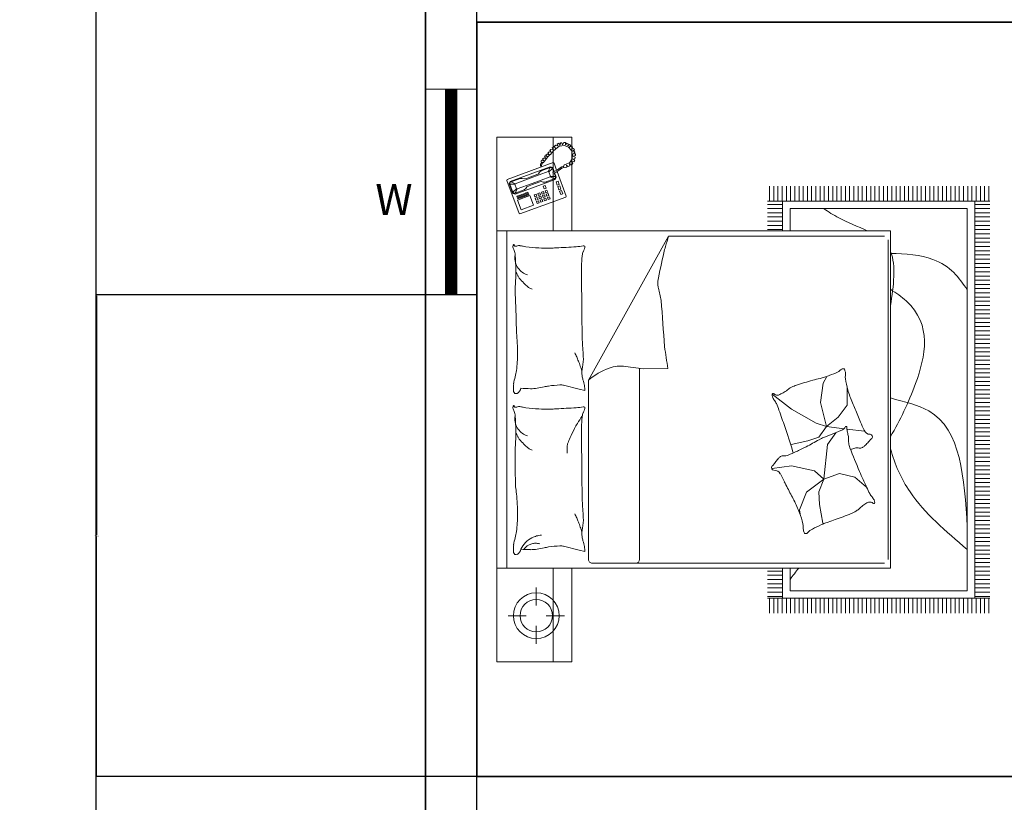
# Model space of a CAD drawing. Units: inches. Extents: x 318 to 927, y -1130 to 13.
# Tile 13 of 17: x 318 to 490, y -297 to -160. Entities that reach past the tile are written whole.
import ezdxf

# ---------------------------------------------------------------- set-up
doc = ezdxf.new("R2010")
doc.units = ezdxf.units.IN
doc.header["$MEASUREMENT"] = 0
for name, color, linetype, lineweight in [('A-ANNO-DIMS', 1, 'Continuous', 18), ('A-ANNO-IDEN', 1, 'Continuous', 13), ('A-GLAZ-PATT', 5, 'Continuous', 9), ('wall', 1, 'Continuous', 35), ('win', 5, 'Continuous', 18)]:
    doc.layers.add(name, color=color, linetype=linetype, lineweight=lineweight)
doc.layers.add('furniture', color=50, linetype='Continuous', lineweight=13, transparency=0.8)
doc.styles.add('DIM_FONT', font='SIMPLEX.shx', dxfattribs={"width": 0.8})
doc.styles.get("Standard").update_dxf_attribs({"font": 'arial.ttf'})
doc.dimstyles.get("Standard").update_dxf_attribs({"dimtxt": 0.18, "dimasz": 0.18, "dimexe": 0.18, "dimexo": 0.0625, "dimgap": 0.09, "dimtad": 0, "dimtih": 1, "dimtoh": 1, "dimdec": 1, "dimzin": 0, "dimdsep": 46, "dimlunit": 4, "dimtxsty": 'Standard', "dimcen": 0.09, "dimadec": 0, "dimazin": 0, "dimtfac": 1, "dimtdec": 1, "dimtofl": 0, "dimtmove": 0, "dimatfit": 3, "dimfxl": 1, "dimtolj": 1, "dimtzin": 0, "dimarcsym": 0})

# ---------------------------------------------------------------- blocks, each defined once
blk = doc.blocks.new('A$C4F634EDD')
for p, q in [((0, 2.6295), (0, 2.2295)), ((0.5, 2.6295), (0, 2.6295)), ((0.5, 2.6295), (2.3, 2.6295)), ((0.5, 0.5295), (0.5, 2.6295)), ((0.5, 2.2295), (0.5, 2.6295)), ((2.3, 2.6295), (2.3, 0.5295)), ((2.3, 2.6295), (2.8, 2.6295)), ((2.3, 2.2295), (2.3, 2.6295)), ((2.8, 2.6295), (2.8, 2.2295)), ((0.5, 2.5771), (2.3, 2.5771)), ((2.392, 2.5115), (2.5692, 2.5765)), ((2.5692, 2.5765), (2.574, 2.5743)), ((2.574, 2.5743), (2.6638, 2.3298)), ((0.2457, 2.5697), (0.2457, 2.4733)), ((2.4842, 2.5232), (2.47, 2.518)), ((2.4862, 2.5179), (2.4842, 2.5232)), ((2.4946, 2.5331), (2.4985, 2.5445)), ((2.5734, 2.3187), (2.4946, 2.5331)), ((2.4985, 2.5445), (2.5516, 2.564)), ((2.5062, 2.5454), (2.5004, 2.5392)), ((2.5004, 2.5392), (2.5013, 2.5315)), ((2.5013, 2.5315), (2.5188, 2.4836)), ((2.5013, 2.5315), (2.5231, 2.5214)), ((2.5062, 2.5454), (2.5487, 2.561)), ((2.5235, 2.5256), (2.5062, 2.5454)), ((2.5231, 2.5214), (2.5235, 2.5256)), ((2.5483, 2.5347), (2.5235, 2.5256)), ((2.5483, 2.5347), (2.5487, 2.561)), ((2.5514, 2.5318), (2.5483, 2.5347)), ((2.5487, 2.561), (2.5571, 2.56)), ((2.5615, 2.5536), (2.5514, 2.5318)), ((2.5807, 2.4521), (2.5514, 2.5318)), ((2.5516, 2.564), (2.5637, 2.5584)), ((2.5571, 2.56), (2.5615, 2.5536)), ((2.5615, 2.5536), (2.5791, 2.5058)), ((2.5637, 2.5584), (2.6418, 2.3458)), ((2.3898, 2.5066), (2.392, 2.5115)), ((2.4795, 2.2621), (2.3898, 2.5066)), ((2.412, 2.5007), (2.4634, 2.5196)), ((2.4361, 2.4352), (2.412, 2.5007)), ((2.4634, 2.5196), (2.4875, 2.454)), ((2.47, 2.518), (2.472, 2.5127)), ((2.472, 2.5127), (2.4862, 2.5179)), ((2.4881, 2.5126), (2.4739, 2.5074)), ((2.4739, 2.5074), (2.4759, 2.502)), ((2.4759, 2.502), (2.4901, 2.5073)), ((2.492, 2.5019), (2.4778, 2.4967)), ((2.4778, 2.4967), (2.4798, 2.4914)), ((2.4798, 2.4914), (2.494, 2.4966)), ((2.4959, 2.4913), (2.4817, 2.4861)), ((2.4817, 2.4861), (2.4837, 2.4808)), ((2.4837, 2.4808), (2.4979, 2.486)), ((2.4998, 2.4807), (2.4856, 2.4755)), ((2.4856, 2.4755), (2.4876, 2.4702)), ((2.4876, 2.4702), (2.5018, 2.4754)), ((2.4901, 2.5073), (2.4881, 2.5126)), ((2.5037, 2.47), (2.4895, 2.4648)), ((2.494, 2.4966), (2.492, 2.5019)), ((2.4979, 2.486), (2.4959, 2.4913)), ((2.5018, 2.4754), (2.4998, 2.4807)), ((2.5057, 2.4647), (2.5037, 2.47)), ((2.5188, 2.4836), (2.5256, 2.4761)), ((2.5523, 2.4417), (2.5231, 2.5214)), ((2.5256, 2.4761), (2.5342, 2.4692)), ((2.5342, 2.4692), (2.5405, 2.4574)), ((2.5788, 2.4956), (2.5767, 2.4848)), ((2.5767, 2.4848), (2.5795, 2.4717)), ((2.5791, 2.5058), (2.5788, 2.4956)), ((2.5795, 2.4717), (2.586, 2.454)), ((0.0957, 2.4197), (0.192, 2.4197)), ((0.2994, 2.4197), (0.3957, 2.4197)), ((2.4875, 2.454), (2.4361, 2.4352)), ((2.4457, 2.4146), (2.4563, 2.4185)), ((2.4563, 2.4185), (2.4602, 2.4078)), ((2.4634, 2.4211), (2.474, 2.425)), ((2.4673, 2.4104), (2.4634, 2.4211)), ((2.474, 2.425), (2.4779, 2.4143)), ((2.4811, 2.4276), (2.4917, 2.4315)), ((2.485, 2.4169), (2.4811, 2.4276)), ((2.4956, 2.4208), (2.485, 2.4169)), ((2.4895, 2.4648), (2.4915, 2.4595)), ((2.4915, 2.4595), (2.5057, 2.4647)), ((2.4917, 2.4315), (2.4956, 2.4208)), ((2.5405, 2.4574), (2.547, 2.4397)), ((2.5594, 2.4061), (2.547, 2.4397)), ((2.5523, 2.4417), (2.5875, 2.346)), ((2.5807, 2.4521), (2.6158, 2.3564)), ((2.5984, 2.4204), (2.586, 2.454)), ((2.6047, 2.4086), (2.5984, 2.4204)), ((0.2457, 2.366), (0.2457, 2.2697)), ((2.4496, 2.4039), (2.4457, 2.4146)), ((2.4602, 2.4078), (2.4496, 2.4039)), ((2.4528, 2.3951), (2.4635, 2.399)), ((2.4567, 2.3844), (2.4528, 2.3951)), ((2.4674, 2.3883), (2.4567, 2.3844)), ((2.46, 2.3756), (2.4706, 2.3795)), ((2.4639, 2.365), (2.46, 2.3756)), ((2.4635, 2.399), (2.4674, 2.3883)), ((2.4745, 2.3689), (2.4639, 2.365)), ((2.4779, 2.4143), (2.4673, 2.4104)), ((2.4706, 2.4016), (2.4812, 2.4055)), ((2.4745, 2.3909), (2.4706, 2.4016)), ((2.4706, 2.3795), (2.4745, 2.3689)), ((2.4851, 2.3949), (2.4745, 2.3909)), ((2.4777, 2.3821), (2.4883, 2.386)), ((2.4816, 2.3715), (2.4777, 2.3821)), ((2.4812, 2.4055), (2.4851, 2.3949)), ((2.4922, 2.3754), (2.4816, 2.3715)), ((2.4849, 2.3626), (2.4955, 2.3665)), ((2.4883, 2.4081), (2.4989, 2.412)), ((2.4922, 2.3975), (2.4883, 2.4081)), ((2.4883, 2.386), (2.4922, 2.3754)), ((2.5028, 2.4014), (2.4922, 2.3975)), ((2.4954, 2.3886), (2.5061, 2.3925)), ((2.4993, 2.378), (2.4954, 2.3886)), ((2.4955, 2.3665), (2.4994, 2.3559)), ((2.4989, 2.412), (2.5028, 2.4014)), ((2.51, 2.3819), (2.4993, 2.378)), ((2.5026, 2.3691), (2.5132, 2.373)), ((2.5065, 2.3585), (2.5026, 2.3691)), ((2.5061, 2.3925), (2.51, 2.3819)), ((2.5132, 2.373), (2.5171, 2.3624)), ((2.5238, 2.3769), (2.538, 2.3821)), ((2.5277, 2.3663), (2.5238, 2.3769)), ((2.5419, 2.3715), (2.5277, 2.3663)), ((2.538, 2.3821), (2.5419, 2.3715)), ((2.5622, 2.393), (2.5594, 2.4061)), ((2.5598, 2.372), (2.5601, 2.3822)), ((2.5774, 2.3242), (2.5598, 2.372)), ((2.5601, 2.3822), (2.5622, 2.393)), ((2.6133, 2.4017), (2.6047, 2.4086)), ((2.6201, 2.3941), (2.6133, 2.4017)), ((2.6376, 2.3463), (2.6201, 2.3941)), ((2.6499, 2.3979), (2.6397, 2.3953)), ((2.6417, 2.39), (2.6488, 2.391)), ((2.6488, 2.391), (2.6538, 2.3895)), ((2.6551, 2.397), (2.6499, 2.3979)), ((2.6538, 2.3895), (2.6596, 2.388)), ((2.6627, 2.392), (2.6551, 2.397)), ((2.6596, 2.388), (2.6626, 2.3867)), ((2.6626, 2.3867), (2.6662, 2.388)), ((2.6692, 2.394), (2.6627, 2.392)), ((2.6662, 2.388), (2.6632, 2.3828)), ((2.6632, 2.3828), (2.6736, 2.3744)), ((2.6736, 2.3944), (2.6692, 2.394)), ((2.6765, 2.391), (2.6736, 2.3944)), ((2.6736, 2.3744), (2.6922, 2.3593)), ((2.6742, 2.3795), (2.6765, 2.391)), ((2.6824, 2.3858), (2.6742, 2.3795)), ((2.6873, 2.3815), (2.6824, 2.3858)), ((2.6853, 2.369), (2.6873, 2.3815)), ((2.6946, 2.376), (2.6853, 2.369)), ((2.6995, 2.3713), (2.6946, 2.376)), ((2.695, 2.3603), (2.6995, 2.3713)), ((2.7031, 2.3682), (2.695, 2.3603)), ((2.7096, 2.3616), (2.7031, 2.3682)), ((0, 2.3301), (0.5, 2.3301)), ((2.8, 2.3301), (2.3, 2.3301)), ((2.4672, 2.3561), (2.4778, 2.36)), ((2.4711, 2.3455), (2.4672, 2.3561)), ((2.4817, 2.3494), (2.4711, 2.3455)), ((2.4778, 2.36), (2.4817, 2.3494)), ((2.4888, 2.352), (2.4849, 2.3626)), ((2.4994, 2.3559), (2.4888, 2.352)), ((2.5171, 2.3624), (2.5065, 2.3585)), ((2.561, 2.3141), (2.5433, 2.3076)), ((2.5649, 2.3035), (2.561, 2.3141)), ((2.5855, 2.3131), (2.5734, 2.3187)), ((2.5774, 2.3242), (2.5875, 2.346)), ((2.5818, 2.3178), (2.5774, 2.3242)), ((2.5901, 2.3168), (2.5818, 2.3178)), ((2.6104, 2.3222), (2.5855, 2.3131)), ((2.5875, 2.346), (2.5905, 2.3431)), ((2.5905, 2.3431), (2.5901, 2.3168)), ((2.5901, 2.3168), (2.6097, 2.324)), ((2.6154, 2.3522), (2.5905, 2.3431)), ((2.613, 2.3312), (2.6077, 2.3293)), ((2.6077, 2.3293), (2.6135, 2.3141)), ((2.6192, 2.3174), (2.613, 2.3312)), ((2.6135, 2.3141), (2.6244, 2.2977)), ((2.6153, 2.3261), (2.6327, 2.3324)), ((2.6158, 2.3564), (2.6154, 2.3522)), ((2.6154, 2.3522), (2.6327, 2.3324)), ((2.6376, 2.3463), (2.6158, 2.3564)), ((2.6369, 2.332), (2.6161, 2.3243)), ((2.626, 2.3069), (2.6192, 2.3174)), ((2.6616, 2.3249), (2.6234, 2.3109)), ((2.6327, 2.3324), (2.6385, 2.3386)), ((2.6418, 2.3458), (2.6369, 2.332)), ((2.6385, 2.3386), (2.6376, 2.3463)), ((2.6638, 2.3298), (2.6616, 2.3249)), ((2.6922, 2.3593), (2.7051, 2.3473)), ((2.7051, 2.3473), (2.7079, 2.3475)), ((2.7062, 2.351), (2.7096, 2.3616)), ((2.7147, 2.3578), (2.7062, 2.351)), ((2.7079, 2.3475), (2.7079, 2.3443)), ((2.7079, 2.3443), (2.727, 2.3277)), ((2.7214, 2.3517), (2.7147, 2.3578)), ((2.7196, 2.34), (2.7214, 2.3517)), ((2.7286, 2.3466), (2.7196, 2.34)), ((2.727, 2.3277), (2.7512, 2.2983)), ((2.7346, 2.3423), (2.7286, 2.3466)), ((2.732, 2.3295), (2.7346, 2.3423)), ((2.7423, 2.3345), (2.732, 2.3295)), ((2.7406, 2.3172), (2.7495, 2.325)), ((2.7519, 2.3218), (2.7406, 2.3172)), ((2.7495, 2.325), (2.7423, 2.3345)), ((2.7575, 2.3144), (2.7519, 2.3218)), ((2.7526, 2.3045), (2.7575, 2.3144)), ((0.5953, 2.1912), (0.616, 2.2738)), ((1.4546, 2.1912), (1.4752, 2.2738)), ((2.4844, 2.2599), (2.4795, 2.2621)), ((2.6172, 2.3086), (2.4844, 2.2599)), ((2.5114, 2.2959), (2.4936, 2.2894)), ((2.4936, 2.2894), (2.4976, 2.2788)), ((2.4976, 2.2788), (2.5153, 2.2853)), ((2.5153, 2.2853), (2.5114, 2.2959)), ((2.5362, 2.305), (2.5185, 2.2985)), ((2.5185, 2.2985), (2.5224, 2.2879)), ((2.5224, 2.2879), (2.5401, 2.2944)), ((2.5401, 2.2944), (2.5362, 2.305)), ((2.5433, 2.3076), (2.5472, 2.297)), ((2.5472, 2.297), (2.5649, 2.3035)), ((2.6244, 2.2977), (2.6349, 2.2825)), ((2.6365, 2.2916), (2.626, 2.3069)), ((2.6349, 2.2825), (2.638, 2.273)), ((2.6407, 2.2834), (2.6365, 2.2916)), ((2.6399, 2.2712), (2.6374, 2.2659)), ((2.6374, 2.2659), (2.6398, 2.257)), ((2.638, 2.273), (2.6399, 2.2712)), ((2.6398, 2.257), (2.6509, 2.259)), ((2.6438, 2.2739), (2.6407, 2.2834)), ((2.6509, 2.259), (2.6431, 2.2492)), ((2.6519, 2.2716), (2.6438, 2.2739)), ((2.6535, 2.2628), (2.6519, 2.2716)), ((2.6636, 2.2409), (2.6535, 2.2628)), ((2.756, 2.2695), (2.7459, 2.2483)), ((2.7512, 2.2983), (2.756, 2.2695)), ((2.7622, 2.308), (2.7526, 2.3045)), ((2.7574, 2.2924), (2.7673, 2.2997)), ((2.7687, 2.2905), (2.7574, 2.2924)), ((2.7587, 2.279), (2.7699, 2.2828)), ((2.7708, 2.2725), (2.7587, 2.279)), ((2.759, 2.2637), (2.7706, 2.2643)), ((2.7676, 2.2559), (2.759, 2.2637)), ((2.7673, 2.2997), (2.7622, 2.308)), ((2.7699, 2.2828), (2.7687, 2.2905)), ((2.7706, 2.2643), (2.7708, 2.2725)), ((0, 2.2295), (0.5, 2.2295)), ((2.8, 2.2295), (2.3, 2.2295)), ((2.6431, 2.2492), (2.6473, 2.2398)), ((2.6473, 2.2398), (2.6592, 2.2429)), ((2.6592, 2.2429), (2.6521, 2.2314)), ((2.6521, 2.2314), (2.6598, 2.2248)), ((2.6598, 2.2248), (2.6697, 2.2309)), ((2.6836, 2.2287), (2.6636, 2.2409)), ((2.6697, 2.2309), (2.6684, 2.219)), ((2.6684, 2.219), (2.6761, 2.2145)), ((2.6761, 2.2145), (2.6821, 2.2237)), ((2.6821, 2.2237), (2.6843, 2.2135)), ((2.7063, 2.2256), (2.6836, 2.2287)), ((2.6843, 2.2135), (2.6927, 2.2117)), ((2.6927, 2.2117), (2.6986, 2.222)), ((2.6986, 2.222), (2.7019, 2.2098)), ((2.7019, 2.2098), (2.7102, 2.2104)), ((2.7284, 2.2317), (2.7063, 2.2256)), ((2.7102, 2.2104), (2.7113, 2.2218)), ((2.7113, 2.2218), (2.7192, 2.2137)), ((2.7192, 2.2137), (2.7255, 2.2152)), ((2.7255, 2.2152), (2.7242, 2.2265)), ((2.7242, 2.2265), (2.7324, 2.2165)), ((2.7459, 2.2483), (2.7284, 2.2317)), ((2.7324, 2.2165), (2.7386, 2.2208)), ((2.7386, 2.2208), (2.7354, 2.2306)), ((2.7354, 2.2306), (2.7462, 2.2264)), ((2.7509, 2.2314), (2.7459, 2.2418)), ((2.7459, 2.2418), (2.7568, 2.2352)), ((2.7462, 2.2264), (2.7509, 2.2314)), ((2.7529, 2.2505), (2.7645, 2.2498)), ((2.7607, 2.2424), (2.7529, 2.2505)), ((2.7568, 2.2352), (2.7607, 2.2424)), ((2.7645, 2.2498), (2.7676, 2.2559)), ((0.5878, 2.1612), (0.5953, 2.1912)), ((1.4471, 2.1612), (1.4546, 2.1912)), ((0.5258, 2.121), (0.5258, 0.5617)), ((1.5035, 2.141), (0.5458, 2.141)), ((1.5035, 2.141), (2.2716, 1.7136)), ((1.576, 1.9433), (1.5624, 1.8479)), ((0.5458, 1.8684), (1.5653, 1.8684)), ((1.5624, 1.8479), (1.5641, 1.7178)), ((2.2716, 0.5617), (2.2716, 1.7136)), ((0.2586, 1.1753), (0.3386, 1.1753)), ((0.3386, 0), (0.3386, 1.1852)), ((0.3486, 1.1052), (0.3486, 1.1852)), ((0.3711, 1.1052), (0.3711, 1.1852)), ((0.3936, 1.1052), (0.3936, 1.1852)), ((0.4161, 1.1052), (0.4161, 1.1852)), ((0.4386, 1.1052), (0.4386, 1.1852)), ((0.4611, 1.1052), (0.4611, 1.1852)), ((0.4836, 1.1052), (0.4836, 1.1852)), ((1.031, 1.1612), (1.0448, 1.0581)), ((1.4276, 1.1611), (1.3484, 1.0571)), ((2.3061, 1.1052), (2.3061, 1.1852)), ((2.3286, 1.1052), (2.3286, 1.1852)), ((2.3511, 1.1052), (2.3511, 1.1852)), ((2.3736, 1.1052), (2.3736, 1.1852)), ((2.3961, 1.1052), (2.3961, 1.1852)), ((2.4186, 1.1052), (2.4186, 1.1852)), ((2.4411, 1.1052), (2.4411, 1.1852)), ((2.4588, 1.1852), (2.4588, 0)), ((2.4588, 1.1753), (2.5388, 1.1753)), ((0.2586, 1.1528), (0.3386, 1.1528)), ((0.2586, 1.1303), (0.3386, 1.1303)), ((0.2586, 1.1078), (0.3386, 1.1078)), ((0.3386, 1.1052), (0.5, 1.1052)), ((2.3, 1.1052), (2.4588, 1.1052)), ((2.4588, 1.1528), (2.5388, 1.1528)), ((2.4588, 1.1303), (2.5388, 1.1303)), ((2.4588, 1.1078), (2.5388, 1.1078)), ((0.2586, 1.0853), (0.3386, 1.0853)), ((0.2586, 1.0628), (0.3386, 1.0628)), ((0.3786, 1.0652), (0.5, 1.0652)), ((0.3786, 0.12), (0.3786, 1.0652)), ((1.0448, 1.0581), (1.019, 0.936)), ((1.1784, 0.9702), (1.1586, 1.0591)), ((1.3484, 1.0571), (1.2733, 0.9268)), ((2.3, 1.0652), (2.4188, 1.0652)), ((2.4188, 1.0652), (2.4188, 0.12)), ((2.4588, 1.0853), (2.5388, 1.0853)), ((2.4588, 1.0628), (2.5388, 1.0628)), ((0.2586, 1.0403), (0.3386, 1.0403)), ((0.2586, 1.0178), (0.3386, 1.0178)), ((0.8108, 1.0151), (0.7868, 1.0117)), ((0.9054, 0.9773), (0.8108, 1.0151)), ((2.4588, 1.0403), (2.5388, 1.0403)), ((2.4588, 1.0178), (2.5388, 1.0178)), ((0.2586, 0.9953), (0.3386, 0.9953)), ((0.2586, 0.9728), (0.3386, 0.9728)), ((0.2586, 0.9503), (0.3386, 0.9503)), ((0.9743, 0.8845), (0.9054, 0.9773)), ((1.1982, 0.9129), (1.1784, 0.9702)), ((2.4588, 0.9953), (2.5388, 0.9953)), ((2.4588, 0.9728), (2.5388, 0.9728)), ((2.4588, 0.9503), (2.5388, 0.9503)), ((0.2586, 0.9278), (0.3386, 0.9278)), ((0.2586, 0.9053), (0.3386, 0.9053)), ((0.8384, 0.9085), (0.7403, 0.8913)), ((0.9072, 0.912), (0.8384, 0.9085)), ((0.9743, 0.8845), (0.9072, 0.912)), ((1.019, 0.936), (0.9743, 0.8845)), ((1.2555, 0.8715), (1.1982, 0.9129)), ((1.2733, 0.9268), (1.2555, 0.8715)), ((1.2555, 0.8715), (1.384, 0.9031)), ((1.384, 0.9031), (1.4868, 0.8892)), ((2.4588, 0.9278), (2.5388, 0.9278)), ((2.4588, 0.9053), (2.5388, 0.9053)), ((0.2586, 0.8828), (0.3386, 0.8828)), ((0.2586, 0.8603), (0.3386, 0.8603)), ((0.7403, 0.8913), (0.737, 0.8849)), ((0.9743, 0.8845), (1.0052, 0.802)), ((0.9743, 0.8845), (1.16, 0.8656)), ((1.16, 0.8656), (1.2099, 0.8295)), ((1.1973, 0.8853), (1.2203, 0.829)), ((1.2555, 0.8715), (1.2437, 0.7773)), ((1.2555, 0.8715), (1.3049, 0.8082)), ((1.4868, 0.8892), (1.5228, 0.8692)), ((2.4588, 0.8828), (2.5388, 0.8828)), ((2.4588, 0.8603), (2.5388, 0.8603)), ((0.2586, 0.8378), (0.3386, 0.8378)), ((0.2586, 0.8153), (0.3386, 0.8153)), ((0.2586, 0.7928), (0.3386, 0.7928)), ((1.0052, 0.802), (0.9846, 0.7194)), ((1.2099, 0.8295), (1.222, 0.8209)), ((1.2203, 0.829), (1.2381, 0.7855)), ((1.3049, 0.8082), (1.3701, 0.7608)), ((2.4588, 0.8378), (2.5388, 0.8378)), ((2.4588, 0.8153), (2.5388, 0.8153)), ((2.4588, 0.7928), (2.5388, 0.7928)), ((0.2586, 0.7703), (0.3386, 0.7703)), ((0.2586, 0.7478), (0.3386, 0.7478)), ((1.2419, 0.7626), (1.23, 0.668)), ((1.3701, 0.7608), (1.463, 0.7608)), ((2.4588, 0.7703), (2.5388, 0.7703)), ((2.4588, 0.7478), (2.5388, 0.7478)), ((0.2586, 0.7253), (0.3386, 0.7253)), ((0.2586, 0.7028), (0.3386, 0.7028)), ((0.9846, 0.7194), (0.931, 0.6569)), ((2.4588, 0.7253), (2.5388, 0.7253)), ((2.4588, 0.7028), (2.5388, 0.7028)), ((0.2586, 0.6803), (0.3386, 0.6803)), ((0.2586, 0.6578), (0.3386, 0.6578)), ((0.2586, 0.6353), (0.3386, 0.6353)), ((2.4588, 0.6803), (2.5388, 0.6803)), ((2.4588, 0.6578), (2.5388, 0.6578)), ((2.4588, 0.6353), (2.5388, 0.6353)), ((0.2586, 0.6128), (0.3386, 0.6128)), ((0.2586, 0.5903), (0.3386, 0.5903)), ((2.4588, 0.6128), (2.5388, 0.6128)), ((2.4588, 0.5903), (2.5388, 0.5903)), ((0.2586, 0.5678), (0.3386, 0.5678)), ((0.2586, 0.5453), (0.3386, 0.5453)), ((2.3, 0.5295), (0.5, 0.5295)), ((0.5458, 0.5417), (2.2516, 0.5417)), ((2.4588, 0.5678), (2.5388, 0.5678)), ((2.4588, 0.5453), (2.5388, 0.5453)), ((0.2586, 0.5228), (0.3386, 0.5228)), ((0.2586, 0.5003), (0.3386, 0.5003)), ((0.2586, 0.4778), (0.3386, 0.4778)), ((2.4588, 0.5228), (2.5388, 0.5228)), ((2.4588, 0.5003), (2.5388, 0.5003)), ((2.4588, 0.4778), (2.5388, 0.4778)), ((0.2586, 0.4553), (0.3386, 0.4553)), ((0.2586, 0.4328), (0.3386, 0.4328)), ((2.4588, 0.4553), (2.5388, 0.4553)), ((2.4588, 0.4328), (2.5388, 0.4328)), ((0.2586, 0.4103), (0.3386, 0.4103)), ((0.2586, 0.3878), (0.3386, 0.3878)), ((2.4588, 0.4103), (2.5388, 0.4103)), ((2.4588, 0.3878), (2.5388, 0.3878)), ((0.2586, 0.3653), (0.3386, 0.3653)), ((0.2586, 0.3428), (0.3386, 0.3428)), ((0.2586, 0.3203), (0.3386, 0.3203)), ((2.4588, 0.3653), (2.5388, 0.3653)), ((2.4588, 0.3428), (2.5388, 0.3428)), ((2.4588, 0.3203), (2.5388, 0.3203)), ((0.2586, 0.2978), (0.3386, 0.2978)), ((0.2586, 0.2753), (0.3386, 0.2753)), ((2.4588, 0.2978), (2.5388, 0.2978)), ((2.4588, 0.2753), (2.5388, 0.2753)), ((0.2586, 0.2528), (0.3386, 0.2528)), ((0.2586, 0.2303), (0.3386, 0.2303)), ((2.4588, 0.2528), (2.5388, 0.2528)), ((2.4588, 0.2303), (2.5388, 0.2303)), ((0.2586, 0.2078), (0.3386, 0.2078)), ((0.2586, 0.1853), (0.3386, 0.1853)), ((0.2586, 0.1628), (0.3386, 0.1628)), ((2.4588, 0.2078), (2.5388, 0.2078)), ((2.4588, 0.1853), (2.5388, 0.1853)), ((2.4588, 0.1628), (2.5388, 0.1628)), ((0.2586, 0.1403), (0.3386, 0.1403)), ((0.2586, 0.1178), (0.3386, 0.1178)), ((2.4188, 0.12), (0.3786, 0.12)), ((2.4588, 0.1403), (2.5388, 0.1403)), ((2.4588, 0.1178), (2.5388, 0.1178)), ((0.2586, 0.0953), (0.3386, 0.0953)), ((0.2586, 0.0728), (0.3386, 0.0728)), ((2.4588, 0.08), (0.3386, 0.08)), ((0.3486, 0), (0.3486, 0.08)), ((0.3711, 0), (0.3711, 0.08)), ((0.3936, 0), (0.3936, 0.08)), ((0.4161, 0), (0.4161, 0.08)), ((0.4386, 0), (0.4386, 0.08)), ((0.4611, 0), (0.4611, 0.08)), ((0.4836, 0), (0.4836, 0.08)), ((0.5061, 0), (0.5061, 0.08)), ((0.5286, 0), (0.5286, 0.08)), ((0.5511, 0), (0.5511, 0.08)), ((0.5736, 0), (0.5736, 0.08)), ((0.5961, 0), (0.5961, 0.08)), ((0.6186, 0), (0.6186, 0.08)), ((0.6411, 0), (0.6411, 0.08)), ((0.6636, 0), (0.6636, 0.08)), ((0.6861, 0), (0.6861, 0.08)), ((0.7086, 0), (0.7086, 0.08)), ((0.7311, 0), (0.7311, 0.08)), ((0.7536, 0), (0.7536, 0.08)), ((0.7761, 0), (0.7761, 0.08)), ((0.7986, 0), (0.7986, 0.08)), ((0.8211, 0), (0.8211, 0.08)), ((0.8436, 0), (0.8436, 0.08)), ((0.8661, 0), (0.8661, 0.08)), ((0.8886, 0), (0.8886, 0.08)), ((0.9111, 0), (0.9111, 0.08)), ((0.9336, 0), (0.9336, 0.08)), ((0.9561, 0), (0.9561, 0.08)), ((0.9786, 0), (0.9786, 0.08)), ((1.0011, 0), (1.0011, 0.08)), ((1.0236, 0), (1.0236, 0.08)), ((1.0461, 0), (1.0461, 0.08)), ((1.0686, 0), (1.0686, 0.08)), ((1.0911, 0), (1.0911, 0.08)), ((1.1136, 0), (1.1136, 0.08)), ((1.1361, 0), (1.1361, 0.08)), ((1.1586, 0), (1.1586, 0.08)), ((1.1811, 0), (1.1811, 0.08)), ((1.2036, 0), (1.2036, 0.08)), ((1.2261, 0), (1.2261, 0.08)), ((1.2486, 0), (1.2486, 0.08)), ((1.2711, 0), (1.2711, 0.08)), ((1.2936, 0), (1.2936, 0.08)), ((1.3161, 0), (1.3161, 0.08)), ((1.3386, 0), (1.3386, 0.08)), ((1.3611, 0), (1.3611, 0.08)), ((1.3836, 0), (1.3836, 0.08)), ((1.4061, 0), (1.4061, 0.08)), ((1.4286, 0), (1.4286, 0.08)), ((1.4511, 0), (1.4511, 0.08)), ((1.4736, 0), (1.4736, 0.08)), ((1.4961, 0), (1.4961, 0.08)), ((1.5186, 0), (1.5186, 0.08)), ((1.5411, 0), (1.5411, 0.08)), ((1.5636, 0), (1.5636, 0.08)), ((1.5861, 0), (1.5861, 0.08)), ((1.6086, 0), (1.6086, 0.08)), ((1.6311, 0), (1.6311, 0.08)), ((1.6536, 0), (1.6536, 0.08)), ((1.6761, 0), (1.6761, 0.08)), ((1.6986, 0), (1.6986, 0.08)), ((1.7211, 0), (1.7211, 0.08)), ((1.7436, 0), (1.7436, 0.08)), ((1.7661, 0), (1.7661, 0.08)), ((1.7886, 0), (1.7886, 0.08)), ((1.8111, 0), (1.8111, 0.08)), ((1.8336, 0), (1.8336, 0.08)), ((1.8561, 0), (1.8561, 0.08)), ((1.8786, 0), (1.8786, 0.08)), ((1.9011, 0), (1.9011, 0.08)), ((1.9236, 0), (1.9236, 0.08)), ((1.9461, 0), (1.9461, 0.08)), ((1.9686, 0), (1.9686, 0.08)), ((1.9911, 0), (1.9911, 0.08)), ((2.0136, 0), (2.0136, 0.08)), ((2.0361, 0), (2.0361, 0.08)), ((2.0586, 0), (2.0586, 0.08)), ((2.0811, 0), (2.0811, 0.08)), ((2.1036, 0), (2.1036, 0.08)), ((2.1261, 0), (2.1261, 0.08)), ((2.1486, 0), (2.1486, 0.08)), ((2.1711, 0), (2.1711, 0.08)), ((2.1936, 0), (2.1936, 0.08)), ((2.2161, 0), (2.2161, 0.08)), ((2.2386, 0), (2.2386, 0.08)), ((2.2611, 0), (2.2611, 0.08)), ((2.2836, 0), (2.2836, 0.08)), ((2.3061, 0), (2.3061, 0.08)), ((2.3286, 0), (2.3286, 0.08)), ((2.3511, 0), (2.3511, 0.08)), ((2.3736, 0), (2.3736, 0.08)), ((2.3961, 0), (2.3961, 0.08)), ((2.4186, 0), (2.4186, 0.08)), ((2.4411, 0), (2.4411, 0.08)), ((2.4588, 0.0953), (2.5388, 0.0953)), ((2.4588, 0.0728), (2.5388, 0.0728)), ((0.2586, 0.0503), (0.3386, 0.0503)), ((0.2586, 0.0278), (0.3386, 0.0278)), ((0.2586, 0.0053), (0.3386, 0.0053)), ((2.4588, 0.0503), (2.5388, 0.0503)), ((2.4588, 0.0278), (2.5388, 0.0278)), ((2.4588, 0.0053), (2.5388, 0.0053))]:
    blk.add_line(p, q)
for radius in [0.1222, 0.0865]:
    blk.add_circle((0.2457, 2.4197), radius)
for centre, radius, start, end in [((0.5848, 2.5274), 0.0131, 101.2724, 206.5805), ((0.5999, 2.4516), 0.0904, 90, 101.2724), ((0.5999, 2.3808), 0.1611, 81.5628, 90), ((0.5788, 2.2388), 0.3048, 74.256, 81.5628), ((0.7272, 2.7653), 0.2422, 254.256, 262.4531), ((0.7851, 3.2019), 0.6827, 262.4531, 270), ((0.7851, 3.5682), 1.049, 270, 276.0867), ((0.8402, 3.0514), 0.5293, 276.0867, 280.1899), ((1.1602, -8.1346), 10.6675, 90.30153, 91.21582), ((1.1169, 2.2433), 0.2897, 85.1982, 92.5386), ((1.2142, 3.4021), 0.8732, 265.1982, 269.4243), ((1.3082, 2.3102), 0.234, 110.8603, 117.2396), ((1.2204, 4.0232), 1.4943, 269.4243, 271.9079), ((1.2995, 2.4357), 0.0992, 105.9352, 126.0864), ((1.2429, 3.3501), 0.8208, 271.9079, 275.2592), ((1.2995, 2.4357), 0.0992, 85.7841, 105.9352), ((1.3132, 2.5864), 0.0539, 275.2592, 300.6513), ((1.3554, 2.5152), 0.0289, 85.6975, 120.6513), ((1.3556, 2.519), 0.0251, 68.2117, 85.6975), ((1.3739, 2.5288), 0.0156, 158.0096, 201.421), ((1.3634, 2.533), 0.00428, 78.1069, 158.0096), ((1.3288, 2.5111), 0.0328, 351.8665, 21.421), ((1.3647, 2.5395), 0.00232, 258.1069, 19.564), ((1.3637, 2.5391), 0.00342, 19.564, 68.2117), ((1.444, 2.5274), 0.0131, 101.2724, 206.5805), ((1.4591, 2.4516), 0.0904, 90, 101.2724), ((1.4591, 2.3808), 0.1611, 81.5628, 90), ((1.438, 2.2388), 0.3048, 74.256, 81.5628), ((1.5865, 2.7653), 0.2422, 254.256, 262.4531), ((1.6443, 3.2019), 0.6827, 262.4531, 270), ((1.6443, 3.5682), 1.049, 270, 276.0867), ((1.4785, 15.4878), 12.9656, 271.22425, 272.05324), ((1.97, 2.3805), 0.1524, 92.5386, 100.1899), ((1.9761, 2.2433), 0.2897, 85.1982, 92.5386), ((2.0734, 3.4021), 0.8732, 265.1982, 269.4243), ((2.1674, 2.3102), 0.234, 110.8603, 117.2396), ((2.0797, 4.0232), 1.4943, 269.4243, 271.9079), ((2.1588, 2.4357), 0.0992, 105.9352, 126.0864), ((2.1021, 3.3501), 0.8208, 271.9079, 275.2592), ((2.1588, 2.4357), 0.0992, 85.7841, 105.9352), ((2.1724, 2.5864), 0.0539, 275.2592, 300.6513), ((2.2146, 2.5152), 0.0289, 85.6975, 120.6513), ((2.2149, 2.519), 0.0251, 68.2117, 85.6975), ((2.2331, 2.5288), 0.0156, 158.0096, 201.421), ((2.2226, 2.533), 0.00428, 78.1069, 158.0096), ((2.1881, 2.5111), 0.0328, 351.8665, 21.421), ((2.224, 2.5395), 0.00232, 258.1069, 19.564), ((2.2229, 2.5391), 0.00342, 19.564, 68.2117), ((0.6036, 2.5368), 0.0342, 206.5805, 265.5998), ((1.0898, 2.4496), 0.4918, 173.7676, 180), ((0.5462, 2.4142), 0.0899, 41.4429, 53.7359), ((0.5368, 2.3783), 0.1399, 45.0976, 62.7964), ((0.5741, 2.4389), 0.0526, 25.3551, 41.4429), ((0.5368, 2.3783), 0.1399, 27.3988, 45.0976), ((1.3165, 2.3233), 0.2252, 133.8115, 140.9651), ((1.4317, 2.2032), 0.3916, 128.3886, 133.8115), ((1.2362, 2.45), 0.0768, 117.2396, 128.3886), ((1.2995, 2.4357), 0.0992, 143.8234, 161.5603), ((1.2995, 2.4357), 0.0992, 126.0864, 143.8234), ((2.2605, 2.3525), 0.9131, 172.3191, 176.6313), ((1.5522, 2.448), 0.1983, 167.8905, 172.3191), ((1.1177, 2.5413), 0.246, 347.8905, 351.8665), ((1.4628, 2.5368), 0.0342, 206.5805, 265.5998), ((1.949, 2.4496), 0.4918, 173.7676, 180), ((2.1757, 2.3233), 0.2252, 133.8115, 140.9651), ((2.291, 2.2032), 0.3916, 128.3886, 133.8115), ((2.0954, 2.45), 0.0768, 117.2396, 128.3886), ((2.1588, 2.4357), 0.0992, 143.8234, 161.5603), ((2.1588, 2.4357), 0.0992, 126.0864, 143.8234), ((3.1198, 2.3525), 0.9131, 172.3191, 176.6313), ((2.4114, 2.448), 0.1983, 167.8905, 172.3191), ((1.977, 2.5413), 0.246, 347.8905, 351.8665), ((0.8019, 2.4496), 0.204, 180, 189.6844), ((0.4851, 2.3967), 0.1511, 21.8149, 25.3551), ((0.4345, 2.3765), 0.2056, 18.7799, 21.8149), ((0.576, 2.4246), 0.0562, 0, 18.7799), ((0.5406, 2.4246), 0.0915, 345.3149, 0), ((0.5368, 2.3783), 0.1399, 16.515, 27.3988), ((0.5368, 2.3783), 0.1399, 5.6311, 16.515), ((1.3127, 2.3625), 0.2002, 151.6832, 156.9972), ((1.1799, 2.4341), 0.0493, 140.9651, 151.6832), ((1.6611, 2.4496), 0.204, 180, 189.6844), ((2.1719, 2.3625), 0.2002, 151.6832, 156.9972), ((2.0391, 2.4341), 0.0493, 140.9651, 151.6832), ((1.4703, 2.5637), 0.882, 189.6844, 192.1984), ((0.2982, 2.3103), 0.3171, 8.0051, 12.1984), ((2.0266, 2.3663), 0.6787, 176.6313, 181.6331), ((2.3295, 2.5637), 0.882, 189.6844, 192.1984), ((1.1575, 2.3103), 0.3171, 8.0051, 12.1984), ((2.8858, 2.3663), 0.6787, 176.6313, 181.6331), ((-0.0401, 2.2627), 0.6588, 2.6649, 8.0051), ((2.7128, 2.3859), 1.3652, 181.6331, 183.055), ((14.9657, 3.0398), 13.6356, 183.05496, 183.50486), ((0.8191, 2.2627), 0.6588, 2.6649, 8.0051), ((3.5721, 2.3859), 1.3652, 181.6331, 183.055), ((15.8249, 3.0398), 13.6356, 183.05496, 183.50486), ((0.5503, 2.2902), 0.0677, 345.9548, 2.6649), ((1.4096, 2.2902), 0.0677, 345.9548, 2.6649), ((0.473, 2.8815), 0.7387, 293.4844, 295.3111), ((1.1303, 1.9835), 0.2721, 85.9172, 93.5552), ((1.1455, 2.197), 0.058, 69.3257, 85.9172), ((0.9871, 1.7772), 0.5066, 65.6735, 69.3257), ((0.6058, 0.9338), 1.4323, 63.5015, 65.6735), ((1.1054, 1.9358), 0.3126, 57.865, 63.5015), ((1.3322, 2.8815), 0.7387, 293.4844, 295.3111), ((0.5887, 2.1609), 0.000917, 165.9551, 274.0829), ((0.5695, 2.4301), 0.2708, 274.0829, 279.4841), ((0.5763, 2.3896), 0.2297, 279.4841, 287.3864), ((0.6807, 2.0561), 0.1197, 96.4341, 107.3864), ((0.6836, 2.0301), 0.1459, 78.4414, 96.4341), ((0.473, 2.8815), 0.7387, 287.1982, 289.428), ((0.759, 2.3985), 0.2301, 258.4414, 272.7491), ((0.473, 2.8815), 0.7387, 289.428, 291.6577), ((0.473, 2.8815), 0.7387, 291.6577, 293.4844), ((0.7026, 3.5718), 1.4048, 272.7491, 274.6176), ((0.9136, 0.9591), 1.2165, 92.6096, 94.6176), ((1.2501, -19.8405), 22.0183, 90.37908, 91.01965), ((1.2012, -3.5404), 5.7185, 89.7135, 90.9704), ((1.224, 1.0141), 1.164, 86.426, 89.7135), ((0.8841, 1.5835), 0.7286, 54.1737, 57.865), ((1.2875, 2.0302), 0.1459, 77.131, 86.426), ((1.3099, 2.1283), 0.0453, 62.7159, 77.131), ((1.3658, 2.2367), 0.0767, 242.7159, 253.7788), ((1.3688, 2.247), 0.0875, 253.7788, 262.8796), ((1.6762, 2.2258), 0.3212, 183.5049, 189.9984), ((1.3581, 2.1615), 0.00132, 262.8796, 343.3022), ((1.3409, 2.1667), 0.0193, 343.3022, 9.9984), ((1.448, 2.1609), 0.000917, 165.9551, 274.0829), ((1.4288, 2.4301), 0.2708, 274.0829, 279.4841), ((1.4355, 2.3896), 0.2297, 279.4841, 287.3864), ((1.5399, 2.0561), 0.1197, 96.4341, 107.3864), ((1.5429, 2.0301), 0.1459, 78.4414, 96.4341), ((1.3322, 2.8815), 0.7387, 287.1982, 289.428), ((1.6182, 2.3985), 0.2301, 258.4414, 272.7491), ((1.3322, 2.8815), 0.7387, 289.428, 291.6577), ((1.3322, 2.8815), 0.7387, 291.6577, 293.4844), ((1.5619, 3.5718), 1.4048, 272.7491, 274.6176), ((1.7729, 0.9591), 1.2165, 92.6096, 94.6176), ((2.1093, -19.8405), 22.0183, 90.37908, 91.01965), ((2.0605, -3.5404), 5.7185, 89.7135, 90.9704), ((2.0833, 1.0141), 1.164, 86.426, 89.7135), ((2.1467, 2.0302), 0.1459, 77.131, 86.426), ((2.1691, 2.1283), 0.0453, 62.7159, 77.131), ((2.2251, 2.2367), 0.0767, 242.7159, 253.7788), ((2.2281, 2.247), 0.0875, 253.7788, 262.8796), ((2.5355, 2.2258), 0.3212, 183.5049, 189.9984), ((2.2174, 2.1615), 0.00132, 262.8796, 343.3022), ((2.2001, 2.1667), 0.0193, 343.3022, 9.9984), ((0.5458, 2.121), 0.02, 90, 180), ((1.2147, 1.9017), 0.3751, 20.1488, 39.6445), ((1.3977, 1.9688), 0.1801, 351.8644, 20.1488), ((0.5458, 1.8884), 0.02, 180, 270), ((1.0582, 5.4638), 3.7801, 277.692, 279.495), ((0.6102, 18.0525), 16.3521, 273.75703, 274.62393), ((1.4194, 4.2174), 2.5158, 281.6741, 283.1904), ((2.0378, 1.5789), 0.1942, 97.7304, 103.1904), ((2.0195, 1.7137), 0.0581, 79.2724, 97.7304), ((1.2737, -2.2227), 4.0646, 77.0745, 79.2724), ((2.0359, 1.0981), 0.6574, 74.0648, 77.0745), ((1.7125, -0.0344), 1.8351, 72.2636, 74.0648), ((1.0348, 1.1521), 0.0127, 51.1864, 183.2455), ((0.9991, 1.1077), 0.0697, 45.8726, 51.1864), ((1.0791, 1.1902), 0.0452, 225.8726, 232.4713), ((1.4338, 1.1026), 0.0601, 110.3452, 128.5854), ((1.4251, 1.1259), 0.0352, 86.0516, 110.3452), ((1.4273, 1.1567), 0.00443, 13.2808, 86.0516), ((1.4254, 1.1562), 0.0063, 306.5792, 13.2808), ((-0.4173, 3.8699), 3.0972, 296.4147, 297.2902), ((0.9863, 1.1494), 0.0359, 297.2902, 3.2455), ((1.2846, 1.4577), 0.3825, 232.4713, 233.7837), ((0.6683, 0.6162), 0.6605, 52.7849, 53.7837), ((0.9362, 0.9689), 0.2176, 46.4776, 52.7849), ((1.0327, 1.0706), 0.0774, 35.8936, 46.4776), ((1.0771, 1.1027), 0.0226, 351.9508, 35.8936), ((-0.4107, 5.9078), 5.0942, 289.0836, 290.1287), ((1.0543, 1.9106), 0.8371, 290.1287, 292.7069), ((1.3469, 1.2115), 0.0792, 292.7069, 308.5854), ((1.4996, 1.1284), 0.0771, 169.5926, 177.2714), ((1.4378, 1.1314), 0.0153, 177.2714, 194.5709), ((1.4611, 1.1374), 0.0393, 194.5709, 206.8179), ((1.4376, 1.1398), 0.0142, 126.5792, 169.5926), ((1.7401, 1.2785), 0.352, 206.8179, 210.9056), ((-1.8336, 6.2238), 5.8383, 297.49208, 297.84822), ((3.744, -4.3336), 6.1019, 117.49986, 117.84822), ((1.8575, -0.7096), 2.0162, 116.4147, 117.4999), ((1.1449, 1.0931), 0.0458, 171.9508, 202.4162), ((2.032, 1.4591), 1.0054, 202.4162, 205.0529), ((1.0922, 1.1636), 0.1166, 280.7366, 286.6085), ((0.2266, 4.0657), 3.145, 286.6085, 289.0836), ((1.6045, 1.1973), 0.194, 210.9056, 219.7005), ((1.3929, 1.0217), 0.081, 26.0735, 39.7005), ((1.2892, 0.9709), 0.1965, 17.8396, 26.0735), ((0.6422, 1.4168), 0.43, 282.6252, 290.7486), ((0.5736, 1.5979), 0.6236, 290.7486, 297.4921), ((2.6493, 1.7476), 1.6868, 205.0529, 207.0884), ((-0.4304, 0.4175), 2.003, 15.2625, 17.8396), ((0.6894, 0.9832), 0.0058, 121.6917, 179.0386), ((0.7004, 0.983), 0.0168, 179.0386, 229.4914), ((0.7131, 0.9448), 0.0509, 103.0402, 121.6917), ((0.6405, 0.9128), 0.0755, 26.3332, 49.4914), ((0.7152, 0.9361), 0.0599, 86.6119, 103.0402), ((-1.6775, -0.2344), 2.6619, 25.1732, 26.3332), ((0.7224, 1.0587), 0.063, 266.6119, 282.6252), ((2.541, 1.6922), 1.5652, 207.0884, 209.936), ((0.5689, 0.8213), 0.1798, 20.7081, 25.1732), ((0.9989, 0.8042), 0.2143, 22.2355, 29.936), ((-0.0881, 0.5109), 1.6481, 13.841, 15.2625), ((2.0418, 1.0357), 0.5454, 193.841, 196.3122), ((0.2268, 0.692), 0.5454, 18.2369, 20.7081), ((2.3102, 1.3785), 1.6481, 198.2369, 199.6584), ((1.6908, 0.933), 0.1798, 196.3122, 200.7773), ((4.0115, 1.8135), 2.6619, 200.7773, 201.9373), ((2.6444, 1.4979), 2.003, 199.6584, 202.2355), ((1.6124, 0.8472), 0.0755, 201.9373, 225.0955), ((1.5473, 0.7819), 0.0168, 354.6428, 45.0955), ((0.9722, 0.8143), 0.1965, 202.2355, 210.4694), ((2.2689, -2.1899), 3.145, 111.0043, 113.4795), ((0.1831, 0.4093), 1.0054, 18.0203, 19.3448), ((1.1834, 0.6373), 0.1166, 98.1216, 111.0043), ((1.1763, 0.687), 0.0663, 85.4882, 98.1216), ((1.1871, 0.8241), 0.0712, 265.4882, 277.6784), ((1.1727, 0.9313), 0.1794, 277.6784, 284.8807), ((1.2689, 0.569), 0.1955, 97.9822, 104.8807), ((1.2594, 0.7942), 0.0231, 202.2355, 252.8133), ((1.2465, 0.729), 0.034, 85.7407, 97.9822), ((1.2497, 0.772), 0.0092, 265.7407, 289.3799), ((1.2512, 0.7678), 0.00467, 289.3799, 72.8133), ((1.6266, 0.159), 0.6236, 106.3527, 113.0962), ((1.5721, 0.3449), 0.43, 98.2293, 106.3527), ((1.5195, 0.708), 0.063, 82.216, 98.2293), ((1.5362, 0.8298), 0.0599, 262.216, 278.6443), ((1.5375, 0.8209), 0.0509, 278.6443, 297.2959), ((1.5582, 0.7808), 0.0058, 297.2959, 354.6428), ((0.8727, 0.7557), 0.081, 210.4694, 224.0964), ((0.6752, 0.5644), 0.194, 35.3015, 44.0964), ((3.0455, -3.9778), 5.0942, 113.4795, 114.5246), ((1.0957, 0.7061), 0.0458, 347.5549, 18.0203), ((1.1625, 0.6914), 0.0226, 167.5549, 211.4977), ((2.4404, -2.1823), 3.0972, 112.0188, 112.8944), ((0.5234, 2.5582), 2.0162, 292.0188, 293.104), ((-1.0798, 6.3161), 6.1019, 293.10398, 293.45234), ((3.6722, -4.6377), 5.8383, 113.0962, 113.45234), ((0.5462, 0.4731), 0.352, 31.2138, 35.3015), ((0.8372, 0.6345), 0.0142, 310.9751, 353.9885), ((0.8136, 0.6351), 0.0393, 18.9668, 31.2138), ((0.8364, 0.6429), 0.0153, 1.6673, 18.9668), ((0.7746, 0.6411), 0.0771, 353.9885, 1.6673), ((0.9332, 0.57), 0.0792, 117.1028, 132.9813), ((1.2784, -0.1047), 0.8371, 114.5246, 117.1028), ((1.2092, 0.72), 0.0774, 211.4977, 222.0817), ((1.3133, 0.814), 0.2176, 222.0817, 228.389), ((1.6074, 1.1451), 0.6605, 228.389, 229.3878), ((0.9284, 0.3533), 0.3825, 48.0754, 49.3878), ((1.1538, 0.6043), 0.0452, 41.4767, 48.0754), ((1.2399, 0.6804), 0.0697, 221.4767, 226.7905), ((1.2009, 0.6389), 0.0127, 226.7905, 358.8496), ((1.2495, 0.6379), 0.0359, 112.8944, 178.8496), ((0.8506, 0.6191), 0.0063, 130.9751, 197.6767), ((0.8488, 0.6185), 0.00443, 197.6767, 270.4475), ((0.8486, 0.6493), 0.0352, 270.4475, 294.7411), ((0.8382, 0.6719), 0.0601, 294.7411, 312.9813)]:
    blk.add_arc(centre, radius, start, end)
for points in [[(0.4393, 1.0652), (0.4595, 1.05), (0.4798, 1.0348), (0.5, 1.0195)], [(1.9003, 0.5295), (2.0065, 0.514), (2.1132, 0.4978), (2.1894, 0.5295)]]:
    blk.add_open_spline(points, degree=3)
for points, knots in [([(2.3, 0.6535), (2.3236, 0.7026), (2.3554, 0.7914), (2.4015, 0.8608), (2.4188, 0.8868)], [1893.525221, 1893.525221, 1893.525221, 1893.525221, 2051.902476, 2146.74457, 2146.74457, 2146.74457, 2146.74457]), ([(0.5992, 0.12), (0.6957, 0.2341), (0.8523, 0.4189), (1.0536, 0.5069), (1.136, 0.5295)], [0, 0, 0, 0, 432.822832, 701.445452, 701.445452, 701.445452, 701.445452]), ([(0.7187, 0.12), (0.9791, 0.1362), (1.326, 0.1577), (1.3868, 0.4574), (1.408, 0.5295)], [0, 0, 0, 0, 653.160442, 870.050857, 870.050857, 870.050857, 870.050857]), ([(1.2016, 0.5295), (1.2892, 0.479), (1.5144, 0.3684), (1.8265, 0.2994), (1.9681, 0.4992), (1.9875, 0.5295)], [936.534237, 936.534237, 936.534237, 936.534237, 1243.285375, 1683.261222, 1758.254386, 1758.254386, 1758.254386, 1758.254386]), ([(2.1796, 0.5295), (2.1798, 0.4519), (2.1548, 0.2369), (2.0487, 0.164), (1.9846, 0.12)], [2202.034493, 2202.034493, 2202.034493, 2202.034493, 2357.807635, 2594.446174, 2594.446174, 2594.446174, 2594.446174])]:
    blk.add_open_spline(points, degree=3, knots=knots)
at = {"style": 'DIM_FONT', "width": 0.8, "flags": 9}
for tag, p in [('YSIZE', (0.5, 2.6295)), ('XSIZE', (0.5, 2.6295)), ('XSIZE', (2.2985, 2.6295)), ('YSIZE', (2.2985, 2.6295))]:
    blk.add_attdef(tag, p, '', height=0.0005, dxfattribs=at)
blk = doc.blocks.new('_ArchTick')
at = {"color": 0, "linetype": 'ByBlock', "const_width": 0.15}
blk.add_lwpolyline([(-0.5, -0.5), (0.5, 0.5)], dxfattribs=at)
blk = doc.blocks.new('*D4')
at = {"layer": 'A-ANNO-DIMS', "color": 0, "lineweight": -2, "transparency": 16777216}
blk.add_line((331.26, -82.91), (331.26, -1042.91), dxfattribs=at)
at = {"layer": 'Defpoints', "color": 0, "transparency": 16777216}
for p in [(388.89, -82.91), (331.26, -1042.91), (388.89, -1042.91)]:
    blk.add_point(p, dxfattribs=at)
at = {"layer": 'A-ANNO-DIMS', "color": 0, "lineweight": -2, "transparency": 16777216, "xscale": 6, "yscale": 6, "zscale": 6}
for p, rotation in [((331.26, -82.91), 90), ((331.26, -1042.91), 270)]:
    blk.add_blockref('_ArchTick', p, dxfattribs=dict(at, rotation=rotation))
at = {"layer": 'A-ANNO-DIMS', "color": 0, "transparency": 16777216, "insert": (323.18, -562.91), "char_height": 8, "attachment_point": 5, "rotation": 90}
blk.add_mtext("\\A1;80'", dxfattribs=at)
blk = doc.blocks.new('WIN-36IN')
for p, q in [((0, 36), (9, 36)), ((3.5, 36), (3.5, 0)), ((5.5, 36), (5.5, 0)), ((0, 0), (9, 0))]:
    blk.add_line(p, q)
blk = doc.blocks.new('*D33')
at = {"layer": 'A-ANNO-DIMS', "color": 0, "lineweight": -2, "transparency": 16777216}
for p, q in [((397.89, -370.85), (397.89, -25.23)), ((398.07, -25.41), (464.5, -25.41)), ((531.71, -25.41), (465.28, -25.41)), ((531.89, -370.85), (531.89, -25.23))]:
    blk.add_line(p, q, dxfattribs=at)
at = {"layer": 'A-ANNO-DIMS', "color": 0, "transparency": 16777216}
for points in [[(398.07, -25.38), (398.07, -25.44), (397.89, -25.41)], [(531.71, -25.38), (531.71, -25.44), (531.89, -25.41)]]:
    blk.add_solid(points, dxfattribs=at)
at = {"layer": 'Defpoints', "color": 0, "transparency": 16777216}
for p in [(531.89, -25.41), (397.89, -370.91), (531.89, -370.91)]:
    blk.add_point(p, dxfattribs=at)
at = {"layer": 'A-ANNO-DIMS', "color": 0, "transparency": 16777216, "insert": (464.89, -25.41), "char_height": 0.18, "attachment_point": 5}
blk.add_mtext('\\A1;11\'-2"', dxfattribs=at)
blk = doc.blocks.new('*D66')
at = {"layer": 'A-ANNO-DIMS', "color": 0, "lineweight": -2, "transparency": 16777216}
for p, q in [((397.83, -208.63), (331.21, -208.63)), ((331.39, -208.81), (331.39, -250.59)), ((331.39, -292.73), (331.39, -250.96)), ((397.83, -292.91), (331.21, -292.91))]:
    blk.add_line(p, q, dxfattribs=at)
at = {"layer": 'A-ANNO-DIMS', "color": 0, "transparency": 16777216}
for points in [[(331.36, -208.81), (331.42, -208.81), (331.39, -208.63)], [(331.36, -292.73), (331.42, -292.73), (331.39, -292.91)]]:
    blk.add_solid(points, dxfattribs=at)
at = {"layer": 'Defpoints', "color": 0, "transparency": 16777216}
for p in [(331.39, -208.63), (397.89, -208.63), (397.89, -292.91)]:
    blk.add_point(p, dxfattribs=at)
at = {"layer": 'A-ANNO-DIMS', "color": 0, "transparency": 16777216, "insert": (331.39, -250.77), "char_height": 0.18, "attachment_point": 5}
blk.add_mtext('\\A1;7\'-0 1/2"', dxfattribs=at)

msp = doc.modelspace()

# ---------------------------------------------------------------- hatches: boundary and pattern name
at = {"layer": 'A-GLAZ-PATT'}
h = msp.add_hatch(dxfattribs=at)
h.set_pattern_fill('ANSI31', color=256)
h.paths.add_polyline_path([(394.39, -636.41), (392.39, -636.41), (392.39, -684.41), (394.39, -684.41)])
h.paths.add_polyline_path([(394.39, -319.91), (392.39, -319.91), (392.39, -343.91), (394.39, -343.91)])
h.paths.add_polyline_path([(394.39, -172.63), (392.39, -172.63), (392.39, -208.63), (394.39, -208.63)])
h.paths.add_polyline_path([(394.39, -109.91), (392.39, -109.91), (392.39, -133.91), (394.39, -133.91)])
h.paths.add_polyline_path([(865.39, -102.49), (863.39, -102.49), (863.39, -138.49), (865.39, -138.49)])

# ---------------------------------------------------------------- linework, layer by layer
at = {"layer": 'wall'}
for p, q in [((388.89, -82.91), (388.89, -1042.91)), ((551.89, -160.91), (397.89, -160.91)), ((397.89, -160.91), (397.89, -292.91)), ((589.89, -292.91), (397.89, -292.91)), ((589.89, -292.91), (397.89, -292.91))]:
    msp.add_line(p, q, dxfattribs=at)

# ---------------------------------------------------------------- block references
at = {"layer": 'furniture', "xscale": 32.78135669785699, "yscale": 32.78135669785699, "zscale": 32.78135669785699, "rotation": 89.99999999999999}
msp.add_blockref('A$C4F634EDD', (487.6, -272.81), dxfattribs=at)
at = {"layer": 'win', "rotation": 180}
msp.add_blockref('WIN-36IN', (397.89, -172.63), dxfattribs=at)

# ---------------------------------------------------------------- texts
at = {"layer": 'A-ANNO-IDEN'}
msp.add_text('W', height=5.44, dxfattribs=at).set_placement((380.13, -194.65))

# ---------------------------------------------------------------- dimensions: what is measured, and where the dimension line sits
at = {"layer": 'A-ANNO-DIMS'}
dim = msp.add_linear_dim(base=(531.89, -25.41), p1=(397.89, -370.91), p2=(531.89, -370.91), dimstyle='Standard', override={"dimdec": 1, "dimlfac": 1, "dimrnd": 0, "dimzin": 1, "dimdsep": 46, "dimlunit": 4, "dimfrac": 2}, dxfattribs=at)
dim.commit()
dim.dimension.update_dxf_attribs({"geometry": '*D33', "text_midpoint": (464.89, -25.41)})
for base, p1, p2, override, picture, middle in [((331.26, -1042.91), (388.89, -82.91), (388.89, -1042.91), {"dimtxt": 8, "dimasz": 6, "dimgap": 4, "dimtad": 1, "dimtih": 0, "dimblk1": 'ArchTick', "dimblk2": 'ArchTick', "dimsah": 1, "dimse1": 1, "dimse2": 1, "dimclrd": 0, "dimclre": 0, "dimclrt": 0}, '*D4', (323.18, -562.91)), ((331.39, -208.63), (397.89, -292.91), (397.89, -208.63), {"dimdec": 1, "dimlfac": 1, "dimrnd": 0, "dimzin": 1, "dimdsep": 46, "dimlunit": 4, "dimfrac": 2}, '*D66', (331.39, -250.77))]:
    dim = msp.add_linear_dim(base=base, p1=p1, p2=p2, angle=90, dimstyle='Standard', override=override, dxfattribs=at)
    dim.commit()
    dim.dimension.update_dxf_attribs({"geometry": picture, "text_midpoint": middle})

doc.saveas('drawing.dxf')
